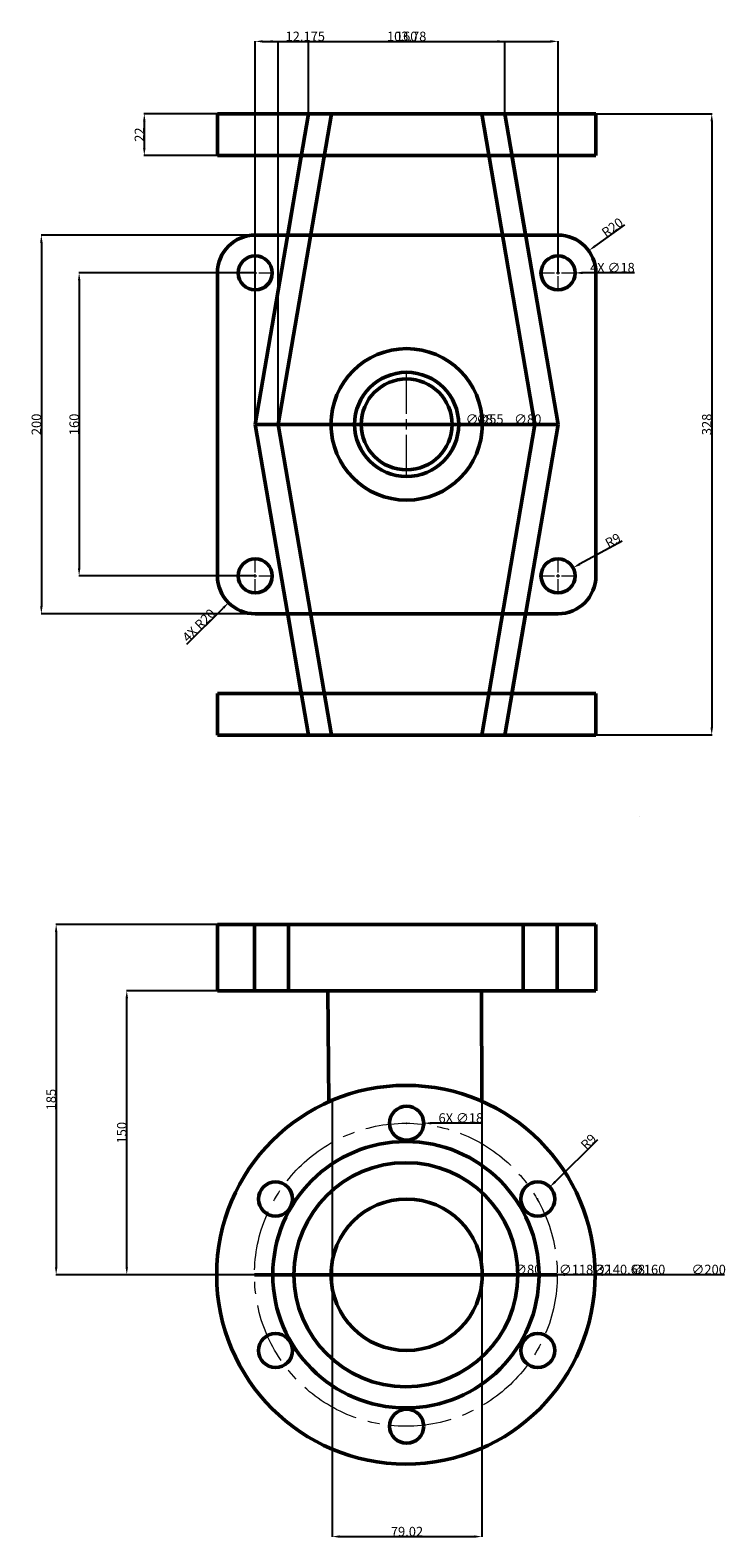
# Model space of a CAD drawing. Units: millimetres. Extents: x 1214 to 1582, y 313 to 1109.
import ezdxf

# ---------------------------------------------------------------- set-up
doc = ezdxf.new("R2010")
doc.units = ezdxf.units.MM
doc.header["$MEASUREMENT"] = 0
doc.linetypes.add('CENTER', pattern=[50.8, 31.75, -6.35, 6.35, -6.35])
for name, color, linetype, lineweight in [('M-CNTR', 1, 'CENTER', 18), ('M-DIMS', 2, 'Continuous', 25), ('M-OUTL', 7, 'Continuous', 50)]:
    doc.layers.add(name, color=color, linetype=linetype, lineweight=lineweight)
doc.styles.get("Standard").update_dxf_attribs({"font": 'arial.ttf'})
doc.dimstyles.get("Standard").update_dxf_attribs({"dimtxt": 5, "dimasz": 4, "dimexe": 0.18, "dimexo": 0.0625, "dimgap": 0.09, "dimtad": 1, "dimdec": 0, "dimzin": 0, "dimdsep": 46, "dimtxsty": 'Standard', "dimcen": 0.09, "dimadec": 0, "dimazin": 0, "dimtfac": 1, "dimtdec": 0, "dimtofl": 0, "dimtmove": 0, "dimatfit": 3, "dimfxl": 1, "dimtolj": 1, "dimtzin": 0, "dimarcsym": 0})

# ---------------------------------------------------------------- blocks, each defined once
blk = doc.blocks.new('*U1')
at = {"layer": 'M-CNTR', "color": 0, "transparency": 16777216}
for p, q in [((0, 1.8), (0, 9.12)), ((-9.12, 0), (-1.8, 0)), ((1.8, 0), (9.12, 0)), ((0, -9.12), (0, -1.8))]:
    blk.add_line(p, q, dxfattribs=at)
at = {"layer": 'M-CNTR', "color": 0, "linetype": 'Continuous', "transparency": 16777216}
for p, q in [((-0.9, 0), (0.9, 0)), ((0, -0.9), (0, 0.9))]:
    blk.add_line(p, q, dxfattribs=at)
blk = doc.blocks.new('*U2')
at = {"layer": 'M-CNTR', "color": 0, "transparency": 16777216}
for p, q in [((0, 1.8), (0, 9.12)), ((-9.12, 0), (-1.8, 0)), ((1.8, 0), (9.12, 0)), ((0, -9.12), (0, -1.8))]:
    blk.add_line(p, q, dxfattribs=at)
at = {"layer": 'M-CNTR', "color": 0, "linetype": 'Continuous', "transparency": 16777216}
for p, q in [((-0.9, 0), (0.9, 0)), ((0, -0.9), (0, 0.9))]:
    blk.add_line(p, q, dxfattribs=at)
blk = doc.blocks.new('*U3')
at = {"layer": 'M-CNTR', "color": 0, "transparency": 16777216}
for p, q in [((0, 1.8), (0, 9.12)), ((-9.12, 0), (-1.8, 0)), ((1.8, 0), (9.12, 0)), ((0, -9.12), (0, -1.8))]:
    blk.add_line(p, q, dxfattribs=at)
at = {"layer": 'M-CNTR', "color": 0, "linetype": 'Continuous', "transparency": 16777216}
for p, q in [((-0.9, 0), (0.9, 0)), ((0, -0.9), (0, 0.9))]:
    blk.add_line(p, q, dxfattribs=at)
blk = doc.blocks.new('*U4')
at = {"layer": 'M-CNTR', "color": 0, "transparency": 16777216}
for p, q in [((0, 1.8), (0, 9.12)), ((-9.12, 0), (-1.8, 0)), ((1.8, 0), (9.12, 0)), ((0, -9.12), (0, -1.8))]:
    blk.add_line(p, q, dxfattribs=at)
at = {"layer": 'M-CNTR', "color": 0, "linetype": 'Continuous', "transparency": 16777216}
for p, q in [((-0.9, 0), (0.9, 0)), ((0, -0.9), (0, 0.9))]:
    blk.add_line(p, q, dxfattribs=at)
blk = doc.blocks.new('*U5')
at = {"layer": 'M-CNTR', "color": 0, "transparency": 16777216}
for p, q in [((0, 5.5), (0, 27.62)), ((-27.62, 0), (-5.5, 0)), ((5.5, 0), (27.62, 0)), ((0, -27.62), (0, -5.5))]:
    blk.add_line(p, q, dxfattribs=at)
at = {"layer": 'M-CNTR', "color": 0, "linetype": 'Continuous', "transparency": 16777216}
for p, q in [((-2.75, 0), (2.75, 0)), ((0, -2.75), (0, 2.75))]:
    blk.add_line(p, q, dxfattribs=at)
blk = doc.blocks.new('*D6')
at = {"layer": 'Defpoints', "color": 0, "transparency": 16777216}
for p in [(1333.05, 981.15), (1239.98, 821.15), (1333.05, 821.15)]:
    blk.add_point(p, dxfattribs=at)
at = {"layer": 'M-DIMS', "color": 0, "lineweight": -2, "transparency": 16777216}
for p, q in [((1332.99, 981.15), (1239.8, 981.15)), ((1239.98, 977.15), (1239.98, 825.15)), ((1332.99, 821.15), (1239.8, 821.15))]:
    blk.add_line(p, q, dxfattribs=at)
at = {"layer": 'M-DIMS', "color": 0, "transparency": 16777216}
for points in [[(1239.32, 977.15), (1240.65, 977.15), (1239.98, 981.15)], [(1239.32, 825.15), (1240.65, 825.15), (1239.98, 821.15)]]:
    blk.add_solid(points, dxfattribs=at)
at = {"layer": 'M-DIMS', "color": 0, "transparency": 16777216, "insert": (1237.34, 901.15), "char_height": 5, "attachment_point": 5, "rotation": 90}
blk.add_mtext('\\A1;160', dxfattribs=at)
blk = doc.blocks.new('*D7')
at = {"layer": 'Defpoints', "color": 0, "transparency": 16777216}
for p in [(1333.05, 1001.15), (1220, 801.15), (1333.05, 801.15)]:
    blk.add_point(p, dxfattribs=at)
at = {"layer": 'M-DIMS', "color": 0, "lineweight": -2, "transparency": 16777216}
for p, q in [((1332.99, 1001.15), (1219.82, 1001.15)), ((1220, 997.15), (1220, 805.15)), ((1332.99, 801.15), (1219.82, 801.15))]:
    blk.add_line(p, q, dxfattribs=at)
at = {"layer": 'M-DIMS', "color": 0, "transparency": 16777216}
for points in [[(1219.33, 997.15), (1220.67, 997.15), (1220, 1001.15)], [(1219.33, 805.15), (1220.67, 805.15), (1220, 801.15)]]:
    blk.add_solid(points, dxfattribs=at)
at = {"layer": 'M-DIMS', "color": 0, "transparency": 16777216, "insert": (1217.36, 901.15), "char_height": 5, "attachment_point": 5, "rotation": 90}
blk.add_mtext('\\A1;200', dxfattribs=at)
blk = doc.blocks.new('*D8')
at = {"layer": 'Defpoints', "color": 0, "transparency": 16777216}
for p in [(1509.26, 992.86), (1493.05, 981.15)]:
    blk.add_point(p, dxfattribs=at)
at = {"layer": 'M-DIMS', "color": 0, "lineweight": -2, "transparency": 16777216}
for p, q in [((1528.24, 1006.58), (1512.5, 995.21)), ((1492.96, 981.15), (1493.14, 981.15)), ((1493.05, 981.06), (1493.05, 981.24))]:
    blk.add_line(p, q, dxfattribs=at)
at = {"layer": 'M-DIMS', "color": 0, "transparency": 16777216}
blk.add_solid([(1512.11, 995.75), (1512.89, 994.67), (1509.26, 992.86)], dxfattribs=at)
at = {"layer": 'M-DIMS', "color": 0, "transparency": 16777216, "insert": (1521.78, 1005.17), "char_height": 5, "attachment_point": 5, "rotation": 35.85966}
blk.add_mtext('\\A1;R20', dxfattribs=at)
blk = doc.blocks.new('*D9')
at = {"layer": 'Defpoints', "color": 0, "transparency": 16777216}
for p in [(1493.05, 821.15), (1500.96, 825.44)]:
    blk.add_point(p, dxfattribs=at)
at = {"layer": 'M-DIMS', "color": 0, "lineweight": -2, "transparency": 16777216}
for p, q in [((1526.96, 839.54), (1504.48, 827.34)), ((1492.96, 821.15), (1493.14, 821.15)), ((1493.05, 821.06), (1493.05, 821.24))]:
    blk.add_line(p, q, dxfattribs=at)
at = {"layer": 'M-DIMS', "color": 0, "transparency": 16777216}
blk.add_solid([(1504.16, 827.93), (1504.8, 826.76), (1500.96, 825.44)], dxfattribs=at)
at = {"layer": 'M-DIMS', "color": 0, "transparency": 16777216, "insert": (1522.07, 839.89), "char_height": 5, "attachment_point": 5, "rotation": 28.47526}
blk.add_mtext('\\A1;R9', dxfattribs=at)
blk = doc.blocks.new('*D10')
at = {"layer": 'Defpoints', "color": 0, "transparency": 16777216}
for p in [(1265.15, 602.15), (1371.32, 602.15), (1373.05, 452.15)]:
    blk.add_point(p, dxfattribs=at)
at = {"layer": 'M-DIMS', "color": 0, "lineweight": -2, "transparency": 16777216}
for p, q in [((1371.26, 602.15), (1264.97, 602.15)), ((1265.15, 456.15), (1265.15, 598.15)), ((1372.99, 452.15), (1264.97, 452.15))]:
    blk.add_line(p, q, dxfattribs=at)
at = {"layer": 'M-DIMS', "color": 0, "transparency": 16777216}
for points in [[(1264.48, 598.15), (1265.81, 598.15), (1265.15, 602.15)], [(1264.48, 456.15), (1265.81, 456.15), (1265.15, 452.15)]]:
    blk.add_solid(points, dxfattribs=at)
at = {"layer": 'M-DIMS', "color": 0, "transparency": 16777216, "insert": (1262.5, 527.15), "char_height": 5, "attachment_point": 5, "rotation": 90}
blk.add_mtext('\\A1;150', dxfattribs=at)
blk = doc.blocks.new('*D11')
at = {"layer": 'Defpoints', "color": 0, "transparency": 16777216}
for p in [(1332.66, 637.15), (1227.83, 452.15), (1332.66, 452.15)]:
    blk.add_point(p, dxfattribs=at)
at = {"layer": 'M-DIMS', "color": 0, "lineweight": -2, "transparency": 16777216}
for p, q in [((1332.6, 637.15), (1227.65, 637.15)), ((1227.83, 633.15), (1227.83, 456.15)), ((1332.6, 452.15), (1227.65, 452.15))]:
    blk.add_line(p, q, dxfattribs=at)
at = {"layer": 'M-DIMS', "color": 0, "transparency": 16777216}
for points in [[(1227.16, 633.15), (1228.49, 633.15), (1227.83, 637.15)], [(1227.16, 456.15), (1228.49, 456.15), (1227.83, 452.15)]]:
    blk.add_solid(points, dxfattribs=at)
at = {"layer": 'M-DIMS', "color": 0, "transparency": 16777216, "insert": (1225.18, 544.65), "char_height": 5, "attachment_point": 5, "rotation": 90}
blk.add_mtext('\\A1;185', dxfattribs=at)
blk = doc.blocks.new('*D12')
at = {"layer": 'Defpoints', "color": 0, "transparency": 16777216}
for p in [(1488.73, 498.47), (1482.33, 492.15)]:
    blk.add_point(p, dxfattribs=at)
at = {"layer": 'M-DIMS', "color": 0, "lineweight": -2, "transparency": 16777216}
for p, q in [((1513.95, 523.4), (1491.58, 501.28)), ((1482.24, 492.15), (1482.42, 492.15)), ((1482.33, 492.06), (1482.33, 492.24))]:
    blk.add_line(p, q, dxfattribs=at)
at = {"layer": 'M-DIMS', "color": 0, "transparency": 16777216}
blk.add_solid([(1491.11, 501.76), (1492.05, 500.81), (1488.73, 498.47)], dxfattribs=at)
at = {"layer": 'M-DIMS', "color": 0, "transparency": 16777216, "insert": (1509.16, 522.38), "char_height": 5, "attachment_point": 5, "rotation": 44.66424}
blk.add_mtext('\\A1;R9', dxfattribs=at)
blk = doc.blocks.new('*D13')
at = {"layer": 'Defpoints', "color": 0, "transparency": 16777216}
for p in [(1493.05, 1103.4), (1333.05, 981.15), (1493.05, 981.15)]:
    blk.add_point(p, dxfattribs=at)
at = {"layer": 'M-DIMS', "color": 0, "lineweight": -2, "transparency": 16777216}
for p, q in [((1333.05, 981.21), (1333.05, 1103.58)), ((1337.05, 1103.4), (1489.05, 1103.4)), ((1493.05, 981.21), (1493.05, 1103.58))]:
    blk.add_line(p, q, dxfattribs=at)
at = {"layer": 'M-DIMS', "color": 0, "transparency": 16777216}
for points in [[(1337.05, 1104.06), (1337.05, 1102.73), (1333.05, 1103.4)], [(1489.05, 1104.06), (1489.05, 1102.73), (1493.05, 1103.4)]]:
    blk.add_solid(points, dxfattribs=at)
at = {"layer": 'M-DIMS', "color": 0, "transparency": 16777216, "insert": (1413.05, 1106.04), "char_height": 5, "attachment_point": 5}
blk.add_mtext('\\A1;160', dxfattribs=at)
blk = doc.blocks.new('*D14')
at = {"layer": 'Defpoints', "color": 0, "transparency": 16777216}
for p in [(1464.94, 1103.4), (1361.16, 1065.15), (1464.94, 1065.15)]:
    blk.add_point(p, dxfattribs=at)
at = {"layer": 'M-DIMS', "color": 0, "lineweight": -2, "transparency": 16777216}
for p, q in [((1361.16, 1065.21), (1361.16, 1103.58)), ((1365.16, 1103.4), (1460.94, 1103.4)), ((1464.94, 1065.21), (1464.94, 1103.58))]:
    blk.add_line(p, q, dxfattribs=at)
at = {"layer": 'M-DIMS', "color": 0, "transparency": 16777216}
for points in [[(1365.16, 1104.06), (1365.16, 1102.73), (1361.16, 1103.4)], [(1460.94, 1104.06), (1460.94, 1102.73), (1464.94, 1103.4)]]:
    blk.add_solid(points, dxfattribs=at)
at = {"layer": 'M-DIMS', "color": 0, "transparency": 16777216, "insert": (1413.05, 1106.04), "char_height": 5, "attachment_point": 5}
blk.add_mtext('\\A1;103.78', dxfattribs=at)
blk = doc.blocks.new('*D15')
at = {"layer": 'Defpoints', "color": 0, "transparency": 16777216}
for p in [(1345.23, 1103.4), (1333.05, 901.15), (1345.23, 901.15)]:
    blk.add_point(p, dxfattribs=at)
at = {"layer": 'M-DIMS', "color": 0, "lineweight": -2, "transparency": 16777216}
for p, q in [((1333.05, 901.21), (1333.05, 1103.58)), ((1337.05, 1103.4), (1341.23, 1103.4)), ((1345.23, 901.21), (1345.23, 1103.58)), ((1345.23, 1103.4), (1369.73, 1103.4))]:
    blk.add_line(p, q, dxfattribs=at)
at = {"layer": 'M-DIMS', "color": 0, "transparency": 16777216}
for points in [[(1337.05, 1104.06), (1337.05, 1102.73), (1333.05, 1103.4)], [(1341.23, 1104.06), (1341.23, 1102.73), (1345.23, 1103.4)]]:
    blk.add_solid(points, dxfattribs=at)
at = {"layer": 'M-DIMS', "color": 0, "transparency": 16777216, "insert": (1359.48, 1106.04), "char_height": 5, "attachment_point": 5}
blk.add_mtext('\\A1;12.175', dxfattribs=at)
blk = doc.blocks.new('*D16')
at = {"layer": 'Defpoints', "color": 0, "transparency": 16777216}
for p in [(1513.05, 1065.15), (1513.05, 737.15), (1574.28, 737.15)]:
    blk.add_point(p, dxfattribs=at)
at = {"layer": 'M-DIMS', "color": 0, "lineweight": -2, "transparency": 16777216}
for p, q in [((1513.11, 1065.15), (1574.46, 1065.15)), ((1574.28, 1061.15), (1574.28, 741.15)), ((1513.11, 737.15), (1574.46, 737.15))]:
    blk.add_line(p, q, dxfattribs=at)
at = {"layer": 'M-DIMS', "color": 0, "transparency": 16777216}
for points in [[(1573.62, 1061.15), (1574.95, 1061.15), (1574.28, 1065.15)], [(1573.62, 741.15), (1574.95, 741.15), (1574.28, 737.15)]]:
    blk.add_solid(points, dxfattribs=at)
at = {"layer": 'M-DIMS', "color": 0, "transparency": 16777216, "insert": (1571.64, 901.15), "char_height": 5, "attachment_point": 5, "rotation": 90}
blk.add_mtext('\\A1;328', dxfattribs=at)
blk = doc.blocks.new('*D17')
at = {"layer": 'Defpoints', "color": 0, "transparency": 16777216}
for p in [(1313.05, 1065.15), (1274.41, 1043.15), (1313.05, 1043.15)]:
    blk.add_point(p, dxfattribs=at)
at = {"layer": 'M-DIMS', "color": 0, "lineweight": -2, "transparency": 16777216}
for p, q in [((1312.99, 1065.15), (1274.23, 1065.15)), ((1274.41, 1061.15), (1274.41, 1047.15)), ((1312.99, 1043.15), (1274.23, 1043.15))]:
    blk.add_line(p, q, dxfattribs=at)
at = {"layer": 'M-DIMS', "color": 0, "transparency": 16777216}
for points in [[(1273.74, 1061.15), (1275.08, 1061.15), (1274.41, 1065.15)], [(1273.74, 1047.15), (1275.08, 1047.15), (1274.41, 1043.15)]]:
    blk.add_solid(points, dxfattribs=at)
at = {"layer": 'M-DIMS', "color": 0, "transparency": 16777216, "insert": (1271.81, 1054.15), "char_height": 5, "attachment_point": 5, "rotation": 90}
blk.add_mtext('\\A1;22', dxfattribs=at)
blk = doc.blocks.new('*D18')
at = {"layer": 'Defpoints', "color": 0, "transparency": 16777216}
for p in [(1373.73, 544.29), (1452.75, 543.76), (1452.75, 313.9)]:
    blk.add_point(p, dxfattribs=at)
at = {"layer": 'M-DIMS', "color": 0, "lineweight": -2, "transparency": 16777216}
for p, q in [((1373.73, 544.23), (1373.73, 313.72)), ((1452.75, 543.69), (1452.75, 313.72)), ((1377.73, 313.9), (1448.75, 313.9))]:
    blk.add_line(p, q, dxfattribs=at)
at = {"layer": 'M-DIMS', "color": 0, "transparency": 16777216}
for points in [[(1377.73, 314.56), (1377.73, 313.23), (1373.73, 313.9)], [(1448.75, 314.56), (1448.75, 313.23), (1452.75, 313.9)]]:
    blk.add_solid(points, dxfattribs=at)
at = {"layer": 'M-DIMS', "color": 0, "transparency": 16777216, "insert": (1413.24, 316.54), "char_height": 5, "attachment_point": 5}
blk.add_mtext('\\A1;79.02', dxfattribs=at)
blk = doc.blocks.new('*D19')
at = {"layer": 'Defpoints', "color": 0, "transparency": 16777216}
for p in [(1312.66, 452.15), (1512.66, 452.15)]:
    blk.add_point(p, dxfattribs=at)
at = {"layer": 'M-DIMS', "color": 0, "lineweight": -2, "transparency": 16777216}
for p, q in [((1412.57, 452.15), (1412.75, 452.15)), ((1412.66, 452.06), (1412.66, 452.24)), ((1580.98, 452.15), (1516.66, 452.15))]:
    blk.add_line(p, q, dxfattribs=at)
at = {"layer": 'M-DIMS', "color": 0, "transparency": 16777216}
blk.add_solid([(1516.66, 452.81), (1516.66, 451.48), (1512.66, 452.15)], dxfattribs=at)
at = {"layer": 'M-DIMS', "color": 0, "transparency": 16777216, "insert": (1572.66, 454.93), "char_height": 5, "attachment_point": 5, "rotation": 359.99988}
blk.add_mtext('\\A1;∅200', dxfattribs=at)
blk = doc.blocks.new('*D20')
at = {"layer": 'Defpoints', "color": 0, "transparency": 16777216}
for p in [(1332.66, 452.15), (1492.66, 452.15)]:
    blk.add_point(p, dxfattribs=at)
at = {"layer": 'M-DIMS', "color": 0, "lineweight": -2, "transparency": 16777216}
for p, q in [((1412.57, 452.15), (1412.75, 452.15)), ((1412.66, 452.06), (1412.66, 452.24)), ((1548.98, 452.15), (1496.66, 452.15))]:
    blk.add_line(p, q, dxfattribs=at)
at = {"layer": 'M-DIMS', "color": 0, "transparency": 16777216}
blk.add_solid([(1496.66, 452.81), (1496.66, 451.48), (1492.66, 452.15)], dxfattribs=at)
at = {"layer": 'M-DIMS', "color": 0, "transparency": 16777216, "insert": (1540.66, 454.93), "char_height": 5, "attachment_point": 5, "rotation": 359.99985}
blk.add_mtext('\\A1;∅160', dxfattribs=at)
blk = doc.blocks.new('*D21')
at = {"layer": 'Defpoints', "color": 0, "transparency": 16777216}
for p in [(1342.32, 452.15), (1483, 452.15)]:
    blk.add_point(p, dxfattribs=at)
at = {"layer": 'M-DIMS', "color": 0, "lineweight": -2, "transparency": 16777216}
for p, q in [((1412.57, 452.15), (1412.75, 452.15)), ((1412.66, 452.06), (1412.66, 452.24)), ((1538.39, 452.15), (1487, 452.15))]:
    blk.add_line(p, q, dxfattribs=at)
at = {"layer": 'M-DIMS', "color": 0, "transparency": 16777216}
blk.add_solid([(1487, 452.81), (1487, 451.48), (1483, 452.15)], dxfattribs=at)
at = {"layer": 'M-DIMS', "color": 0, "transparency": 16777216, "insert": (1525.2, 454.93), "char_height": 5, "attachment_point": 5, "rotation": 359.99982}
blk.add_mtext('\\A1;∅140.68', dxfattribs=at)
blk = doc.blocks.new('*D22')
at = {"layer": 'Defpoints', "color": 0, "transparency": 16777216}
for p in [(1353.5, 452.15), (1471.82, 452.15)]:
    blk.add_point(p, dxfattribs=at)
at = {"layer": 'M-DIMS', "color": 0, "lineweight": -2, "transparency": 16777216}
for p, q in [((1412.57, 452.15), (1412.75, 452.15)), ((1412.66, 452.06), (1412.66, 452.24)), ((1520.48, 452.15), (1475.82, 452.15))]:
    blk.add_line(p, q, dxfattribs=at)
at = {"layer": 'M-DIMS', "color": 0, "transparency": 16777216}
blk.add_solid([(1475.82, 452.81), (1475.82, 451.48), (1471.82, 452.15)], dxfattribs=at)
at = {"layer": 'M-DIMS', "color": 0, "transparency": 16777216, "insert": (1507.31, 454.93), "char_height": 5, "attachment_point": 5, "rotation": 359.99979}
blk.add_mtext('\\A1;∅118.32', dxfattribs=at)
blk = doc.blocks.new('*D23')
at = {"layer": 'Defpoints', "color": 0, "transparency": 16777216}
for p in [(1373.05, 452.15), (1453.05, 452.15)]:
    blk.add_point(p, dxfattribs=at)
at = {"layer": 'M-DIMS', "color": 0, "lineweight": -2, "transparency": 16777216}
for p, q in [((1412.96, 452.15), (1413.14, 452.15)), ((1413.05, 452.06), (1413.05, 452.24)), ((1483.43, 452.15), (1457.05, 452.15))]:
    blk.add_line(p, q, dxfattribs=at)
at = {"layer": 'M-DIMS', "color": 0, "transparency": 16777216}
blk.add_solid([(1457.05, 452.81), (1457.05, 451.48), (1453.05, 452.15)], dxfattribs=at)
at = {"layer": 'M-DIMS', "color": 0, "transparency": 16777216, "insert": (1477.05, 454.93), "char_height": 5, "attachment_point": 5, "rotation": 359.99969}
blk.add_mtext('\\A1;∅80', dxfattribs=at)
blk = doc.blocks.new('*D24')
at = {"layer": 'Defpoints', "color": 0, "transparency": 16777216}
for p in [(1373.05, 901.15), (1453.05, 901.15)]:
    blk.add_point(p, dxfattribs=at)
at = {"layer": 'M-DIMS', "color": 0, "lineweight": -2, "transparency": 16777216}
for p, q in [((1412.96, 901.15), (1413.14, 901.15)), ((1413.05, 901.06), (1413.05, 901.24)), ((1483.43, 901.15), (1457.05, 901.15))]:
    blk.add_line(p, q, dxfattribs=at)
at = {"layer": 'M-DIMS', "color": 0, "transparency": 16777216}
blk.add_solid([(1457.05, 901.81), (1457.05, 900.48), (1453.05, 901.15)], dxfattribs=at)
at = {"layer": 'M-DIMS', "color": 0, "transparency": 16777216, "insert": (1477.05, 903.93), "char_height": 5, "attachment_point": 5, "rotation": 359.99969}
blk.add_mtext('\\A1;∅80', dxfattribs=at)
blk = doc.blocks.new('*D25')
at = {"layer": 'Defpoints', "color": 0, "transparency": 16777216}
for p in [(1385.55, 901.15), (1440.55, 901.15)]:
    blk.add_point(p, dxfattribs=at)
at = {"layer": 'M-DIMS', "color": 0, "lineweight": -2, "transparency": 16777216}
for p, q in [((1412.96, 901.15), (1413.14, 901.15)), ((1413.05, 901.06), (1413.05, 901.24)), ((1463.46, 901.15), (1444.55, 901.15))]:
    blk.add_line(p, q, dxfattribs=at)
at = {"layer": 'M-DIMS', "color": 0, "transparency": 16777216}
blk.add_solid([(1444.55, 901.81), (1444.55, 900.48), (1440.55, 901.15)], dxfattribs=at)
at = {"layer": 'M-DIMS', "color": 0, "transparency": 16777216, "insert": (1457.05, 903.93), "char_height": 5, "attachment_point": 5, "rotation": 359.99955}
blk.add_mtext('\\A1;∅55', dxfattribs=at)
blk = doc.blocks.new('*D26')
at = {"layer": 'Defpoints', "color": 0, "transparency": 16777216}
for p in [(1389.05, 901.15), (1437.05, 901.15)]:
    blk.add_point(p, dxfattribs=at)
at = {"layer": 'M-DIMS', "color": 0, "lineweight": -2, "transparency": 16777216}
for p, q in [((1412.96, 901.15), (1413.14, 901.15)), ((1413.05, 901.06), (1413.05, 901.24)), ((1457.85, 901.15), (1441.05, 901.15))]:
    blk.add_line(p, q, dxfattribs=at)
at = {"layer": 'M-DIMS', "color": 0, "transparency": 16777216}
blk.add_solid([(1441.05, 901.81), (1441.05, 900.48), (1437.05, 901.15)], dxfattribs=at)
at = {"layer": 'M-DIMS', "color": 0, "transparency": 16777216, "insert": (1451.45, 903.93), "char_height": 5, "attachment_point": 5, "rotation": 359.99949}
blk.add_mtext('\\A1;∅48', dxfattribs=at)
blk = doc.blocks.new('*D27')
at = {"layer": 'Defpoints', "color": 0, "transparency": 16777216}
for p in [(1484.05, 981.15), (1502.05, 981.15)]:
    blk.add_point(p, dxfattribs=at)
at = {"layer": 'M-DIMS', "color": 0, "lineweight": -2, "transparency": 16777216}
for p, q in [((1492.96, 981.15), (1493.14, 981.15)), ((1493.05, 981.06), (1493.05, 981.24)), ((1533.52, 981.15), (1506.05, 981.15))]:
    blk.add_line(p, q, dxfattribs=at)
at = {"layer": 'M-DIMS', "color": 0, "transparency": 16777216}
blk.add_solid([(1506.05, 981.81), (1506.05, 980.48), (1502.05, 981.15)], dxfattribs=at)
at = {"layer": 'M-DIMS', "color": 0, "transparency": 16777216, "insert": (1521.79, 983.93), "char_height": 5, "attachment_point": 5, "rotation": 359.99863}
blk.add_mtext('\\A1;4X ∅18', dxfattribs=at)
blk = doc.blocks.new('*D28')
at = {"layer": 'Defpoints', "color": 0, "transparency": 16777216}
for p in [(1333.05, 821.15), (1318.91, 807)]:
    blk.add_point(p, dxfattribs=at)
at = {"layer": 'M-DIMS', "color": 0, "lineweight": -2, "transparency": 16777216}
for p, q in [((1332.96, 821.15), (1333.14, 821.15)), ((1333.05, 821.06), (1333.05, 821.24)), ((1296.95, 785.04), (1316.08, 804.18))]:
    blk.add_line(p, q, dxfattribs=at)
at = {"layer": 'M-DIMS', "color": 0, "transparency": 16777216}
blk.add_solid([(1315.61, 804.65), (1316.55, 803.7), (1318.91, 807)], dxfattribs=at)
at = {"layer": 'M-DIMS', "color": 0, "transparency": 16777216, "insert": (1303.23, 795.06), "char_height": 5, "attachment_point": 5, "rotation": 45.0002}
blk.add_mtext('\\A1;4X R20', dxfattribs=at)
blk = doc.blocks.new('*D29')
at = {"layer": 'Defpoints', "color": 0, "transparency": 16777216}
for p in [(1404.05, 532.14), (1422.05, 532.15)]:
    blk.add_point(p, dxfattribs=at)
at = {"layer": 'M-DIMS', "color": 0, "lineweight": -2, "transparency": 16777216}
for p, q in [((1412.96, 532.15), (1413.14, 532.15)), ((1413.05, 532.06), (1413.05, 532.24)), ((1453.35, 532.17), (1426.05, 532.15))]:
    blk.add_line(p, q, dxfattribs=at)
at = {"layer": 'M-DIMS', "color": 0, "transparency": 16777216}
blk.add_solid([(1426.05, 532.82), (1426.05, 531.49), (1422.05, 532.15)], dxfattribs=at)
at = {"layer": 'M-DIMS', "color": 0, "transparency": 16777216, "insert": (1441.7, 534.94), "char_height": 5, "attachment_point": 5, "rotation": 0.03018}
blk.add_mtext('\\A1;6X ∅18', dxfattribs=at)

msp = doc.modelspace()

# ---------------------------------------------------------------- linework, layer by layer
at = {"layer": 'M-CNTR'}
msp.add_circle((1412.6591, 452.1462), 80, dxfattribs=at)
at = {"layer": 'M-OUTL'}
for p, q in [((1513.0501, 1065.1462), (1313.0501, 1065.1462)), ((1313.0501, 1065.1462), (1313.0501, 1043.1462)), ((1333.0501, 901.1462), (1361.1584, 1065.1462)), ((1345.2251, 901.1462), (1373.3333, 1065.1462)), ((1480.8751, 901.1462), (1452.7669, 1065.1462)), ((1493.0501, 901.1462), (1464.9419, 1065.1462)), ((1513.0501, 1043.1462), (1513.0501, 1065.1462)), ((1313.0501, 1043.1462), (1513.0501, 1043.1462)), ((1357.3878, 1043.1462), (1350.1893, 1001.1462)), ((1468.7125, 1043.1462), (1475.9109, 1001.1462)), ((1413.0501, 901.1462), (1333.0501, 901.1462)), ((1333.0501, 901.1462), (1361.1584, 737.1462)), ((1345.2251, 901.1462), (1373.3333, 737.1462)), ((1413.0501, 901.1462), (1493.0501, 901.1462)), ((1480.8751, 901.1462), (1452.7669, 737.1462)), ((1493.0501, 901.1462), (1464.9419, 737.1462)), ((1413.0501, 801.1462), (1333.0501, 801.1462)), ((1350.1893, 801.1462), (1357.3878, 759.1462)), ((1468.7125, 759.1462), (1475.9109, 801.1462)), ((1513.0501, 759.1462), (1313.0501, 759.1462)), ((1313.0501, 759.1462), (1313.0501, 737.1462)), ((1513.0501, 737.1462), (1513.0501, 759.1462)), ((1313.0501, 737.1462), (1513.0501, 737.1462)), ((1536.0345, 693.9163), (1536.0345, 693.9163)), ((1313.0501, 637.1462), (1313.0501, 602.1462)), ((1332.6591, 637.1462), (1313.0501, 637.1462)), ((1332.6591, 637.1462), (1492.6591, 637.1462)), ((1332.6591, 602.1462), (1332.6591, 637.1462)), ((1332.6591, 637.1462), (1492.6591, 637.1462)), ((1350.6591, 602.1462), (1350.6591, 637.1462)), ((1474.6591, 637.1462), (1474.6591, 602.1462)), ((1492.6591, 637.1462), (1492.6591, 602.1462)), ((1513.0501, 637.1462), (1492.6591, 637.1462)), ((1513.0501, 602.1462), (1513.0501, 637.1462)), ((1313.0501, 602.1462), (1332.6591, 602.1462)), ((1492.6591, 602.1462), (1332.6591, 602.1462)), ((1371.3201, 602.1462), (1371.9911, 543.5033)), ((1452.5624, 602.1462), (1452.5624, 602.1462)), ((1452.5624, 602.1462), (1452.7523, 543.757)), ((1492.6591, 602.1462), (1513.0501, 602.1462)), ((1492.6591, 452.1462), (1332.6591, 452.1462))]:
    msp.add_line(p, q, dxfattribs=at)
msp.add_lwpolyline([(1313.0501, 981.1462, -0.41421356), (1333.0501, 1001.1462), (1493.0501, 1001.1462, -0.41421356), (1513.0501, 981.1462), (1513.0501, 821.1462, -0.41421356), (1493.0501, 801.1462), (1333.0501, 801.1462, -0.41421356), (1313.0501, 821.1462)], format="xyb", close=True, dxfattribs=at)
for centre, radius in [((1333.0501, 981.1462), 9), ((1493.0501, 981.1462), 9), ((1413.0501, 901.1462), 40), ((1413.0501, 901.1462), 27.5), ((1413.0501, 901.1462), 24), ((1333.0501, 821.1462), 9), ((1493.0501, 821.1462), 9), ((1412.6591, 452.1462), 100), ((1413.0501, 532.1453), 9), ((1412.6591, 452.1462), 70.3377), ((1412.6591, 452.1462), 59.1599), ((1343.7689, 492.1457), 9), ((1482.3313, 492.1457), 9), ((1413.0501, 452.1462), 40), ((1343.7689, 412.1467), 9), ((1482.3313, 412.1467), 9), ((1413.0501, 372.1472), 9)]:
    msp.add_circle(centre, radius, dxfattribs=at)

# ---------------------------------------------------------------- block references
at = {"layer": 'M-CNTR'}
for name, p in [('*U1', (1333.0501, 981.1462)), ('*U4', (1493.0501, 981.1462)), ('*U5', (1413.0501, 901.1462)), ('*U2', (1333.0501, 821.1462)), ('*U3', (1493.0501, 821.1462))]:
    msp.add_blockref(name, p, dxfattribs=at)

# ---------------------------------------------------------------- dimensions: what is measured, and where the dimension line sits
at = {"layer": 'M-DIMS'}
for base, p1, p2, override, picture, middle in [((1493.0501, 1103.3962), (1333.0501, 981.1462), (1493.0501, 981.1462), {"dimdec": 0, "dimlfac": 1, "dimrnd": 0, "dimzin": 0, "dimdsep": 46, "dimlunit": 2}, '*D13', (1413.0501, 1106.0391)), ((1345.2251, 1103.3962), (1333.0501, 901.1462), (1345.2251, 901.1462), {"dimdec": 3, "dimlfac": 1, "dimrnd": 0, "dimzin": 0, "dimdsep": 46, "dimlunit": 2}, '*D15', (1359.4771, 1106.0391)), ((1464.9419, 1103.3962), (1361.1584, 1065.1462), (1464.9419, 1065.1462), {"dimdec": 2, "dimlfac": 1, "dimrnd": 0, "dimzin": 0, "dimdsep": 46, "dimlunit": 2}, '*D14', (1413.0501, 1106.0408)), ((1452.7523, 313.8962), (1373.7346, 544.2877), (1452.7523, 543.757), {"dimdec": 2, "dimlfac": 1, "dimrnd": 0, "dimzin": 0, "dimdsep": 46, "dimlunit": 2}, '*D18', (1413.2435, 316.5391))]:
    dim = msp.add_linear_dim(base=base, p1=p1, p2=p2, dimstyle='Standard', override=override, dxfattribs=at)
    dim.commit()
    dim.dimension.update_dxf_attribs({"geometry": picture, "text_midpoint": middle})
for base, p1, p2, override, picture, middle in [((1274.4091, 1043.1462), (1313.0501, 1065.1462), (1313.0501, 1043.1462), {"dimdec": 0, "dimlfac": 1, "dimrnd": 0, "dimzin": 0, "dimdsep": 46, "dimlunit": 2}, '*D17', (1271.8089, 1054.1462)), ((1574.2845, 737.1462), (1513.0501, 1065.1462), (1513.0501, 737.1462), {"dimdec": 0, "dimlfac": 1, "dimrnd": 0, "dimzin": 0, "dimdsep": 46, "dimlunit": 2}, '*D16', (1571.6399, 901.1462)), ((1219.9988, 801.1462), (1333.0501, 1001.1462), (1333.0501, 801.1462), {"dimclrd": 0, "dimclre": 0, "dimclrt": 0}, '*D7', (1217.3559, 901.1462)), ((1239.9837, 821.1462), (1333.0501, 981.1462), (1333.0501, 821.1462), {"dimclrd": 0, "dimclre": 0, "dimclrt": 0}, '*D6', (1237.3408, 901.1462)), ((1227.8272, 452.1462), (1332.6591, 637.1462), (1332.6591, 452.1462), {"dimclrd": 0, "dimclre": 0, "dimclrt": 0}, '*D11', (1225.1843, 544.6462)), ((1265.1463, 602.1462), (1373.0501, 452.1462), (1371.3201, 602.1462), {"dimclrd": 0, "dimclre": 0, "dimclrt": 0}, '*D10', (1262.5034, 527.1462))]:
    dim = msp.add_linear_dim(base=base, p1=p1, p2=p2, angle=90, dimstyle='Standard', override=override, dxfattribs=at)
    dim.commit()
    dim.dimension.update_dxf_attribs({"geometry": picture, "text_midpoint": middle})
for center, mpoint, picture, middle in [((1493.0501, 981.1462), (1509.2592, 992.8623), '*D8', (1523.3295, 1003.0324)), ((1493.0501, 821.1462), (1500.9613, 825.4372), '*D9', (1523.3295, 837.5697)), ((1482.3313, 492.1457), (1488.7325, 498.4723), '*D12', (1511.0172, 520.4974))]:
    dim = msp.add_radius_dim(center=center, mpoint=mpoint, dimstyle='Standard', override={"dimclrd": 0, "dimclre": 0, "dimclrt": 0}, dxfattribs=at)
    dim.commit()
    dim.dimension.update_dxf_attribs({"geometry": picture, "text_midpoint": middle, "dimtype": 164})
dim = msp.add_diameter_dim_2p(p1=(1484.0501, 981.1464), p2=(1502.0501, 981.146), text='4X <>', dimstyle='Standard', override={"dimdec": 0, "dimlfac": 1, "dimrnd": 0, "dimzin": 0, "dimdsep": 46, "dimlunit": 2}, dxfattribs=at)
dim.commit()
dim.dimension.update_dxf_attribs({"geometry": '*D27', "text_midpoint": (1521.7858, 981.1455)})
for p1, p2, override, picture, middle in [((1373.0501, 901.1464), (1453.0501, 901.146), {"dimdec": 0, "dimlfac": 1, "dimrnd": 0, "dimzin": 0, "dimdsep": 46, "dimlunit": 2}, '*D24', (1477.0501, 901.1459)), ((1385.5501, 901.1464), (1440.5501, 901.146), {"dimdec": 0, "dimlfac": 1, "dimrnd": 0, "dimzin": 0, "dimdsep": 46, "dimlunit": 2}, '*D25', (1457.0501, 901.1459)), ((1389.0501, 901.1464), (1437.0501, 901.146), {"dimdec": 0, "dimlfac": 1, "dimrnd": 0, "dimzin": 0, "dimdsep": 46, "dimlunit": 2}, '*D26', (1451.4501, 901.1459)), ((1312.6591, 452.1464), (1512.6591, 452.146), {"dimdec": 0, "dimlfac": 1, "dimrnd": 0, "dimzin": 0, "dimdsep": 46, "dimlunit": 2}, '*D19', (1572.6591, 452.1459)), ((1332.6591, 452.1464), (1492.6591, 452.146), {"dimdec": 0, "dimlfac": 1, "dimrnd": 0, "dimzin": 0, "dimdsep": 46, "dimlunit": 2}, '*D20', (1540.6591, 452.1459)), ((1342.3214, 452.1464), (1482.9969, 452.146), {"dimdec": 2, "dimlfac": 1, "dimrnd": 0, "dimzin": 0, "dimdsep": 46, "dimlunit": 2}, '*D21', (1525.1995, 452.1459)), ((1353.4992, 452.1464), (1471.819, 452.146), {"dimdec": 2, "dimlfac": 1, "dimrnd": 0, "dimzin": 0, "dimdsep": 46, "dimlunit": 2}, '*D22', (1507.315, 452.1459)), ((1373.0501, 452.1464), (1453.0501, 452.146), {"dimdec": 0, "dimlfac": 1, "dimrnd": 0, "dimzin": 0, "dimdsep": 46, "dimlunit": 2}, '*D23', (1477.0501, 452.1459))]:
    dim = msp.add_diameter_dim_2p(p1=p1, p2=p2, dimstyle='Standard', override=override, dxfattribs=at)
    dim.commit()
    dim.dimension.update_dxf_attribs({"geometry": picture, "text_midpoint": middle, "dimtype": 163})
dim = msp.add_radius_dim(center=(1333.0501, 821.1462), mpoint=(1318.908, 807.004), text='4X <>', dimstyle='Standard', override={"dimdec": 0, "dimlfac": 1, "dimrnd": 0, "dimzin": 0, "dimdsep": 46, "dimlunit": 2}, dxfattribs=at)
dim.commit()
dim.dimension.update_dxf_attribs({"geometry": '*D28', "text_midpoint": (1303.2312, 795.0647)})
dim = msp.add_diameter_dim_2p(p1=(1404.0501, 532.1405), p2=(1422.0501, 532.15), text='6X <>', dimstyle='Standard', override={"dimdec": 0, "dimlfac": 1, "dimrnd": 0, "dimzin": 0, "dimdsep": 46, "dimlunit": 2}, dxfattribs=at)
dim.commit()
dim.dimension.update_dxf_attribs({"geometry": '*D29', "text_midpoint": (1441.6988, 532.1604), "dimtype": 163})

doc.saveas('drawing.dxf')
